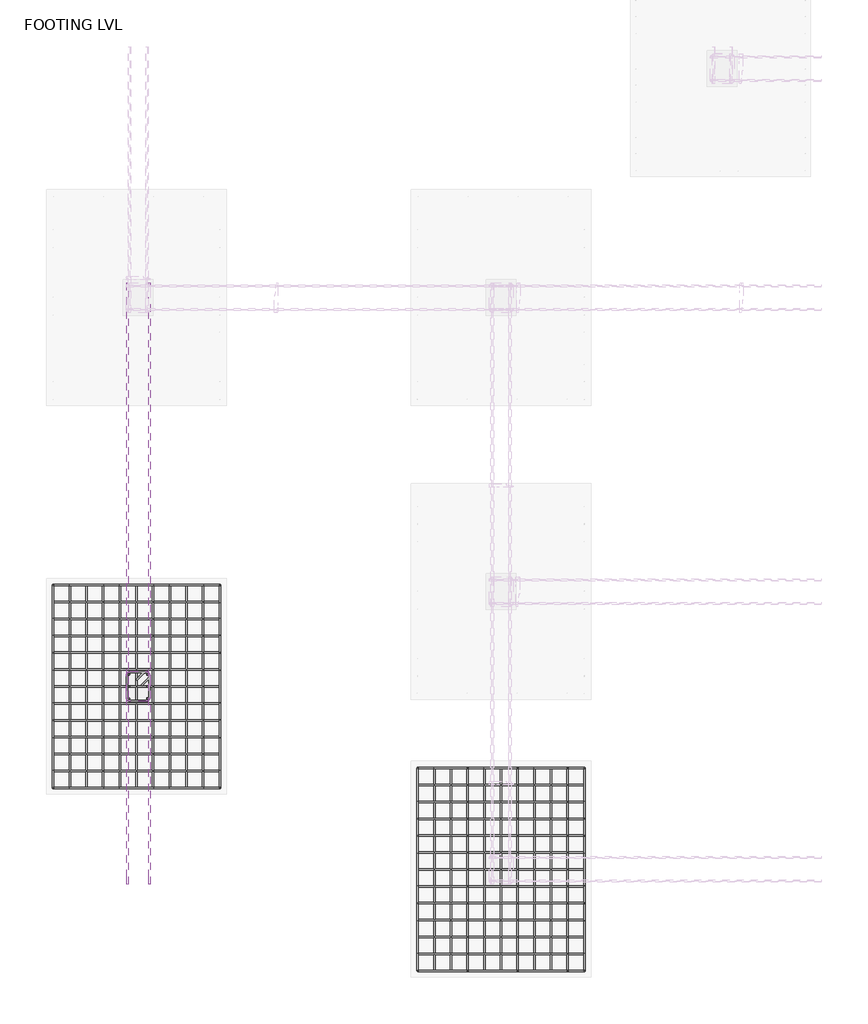
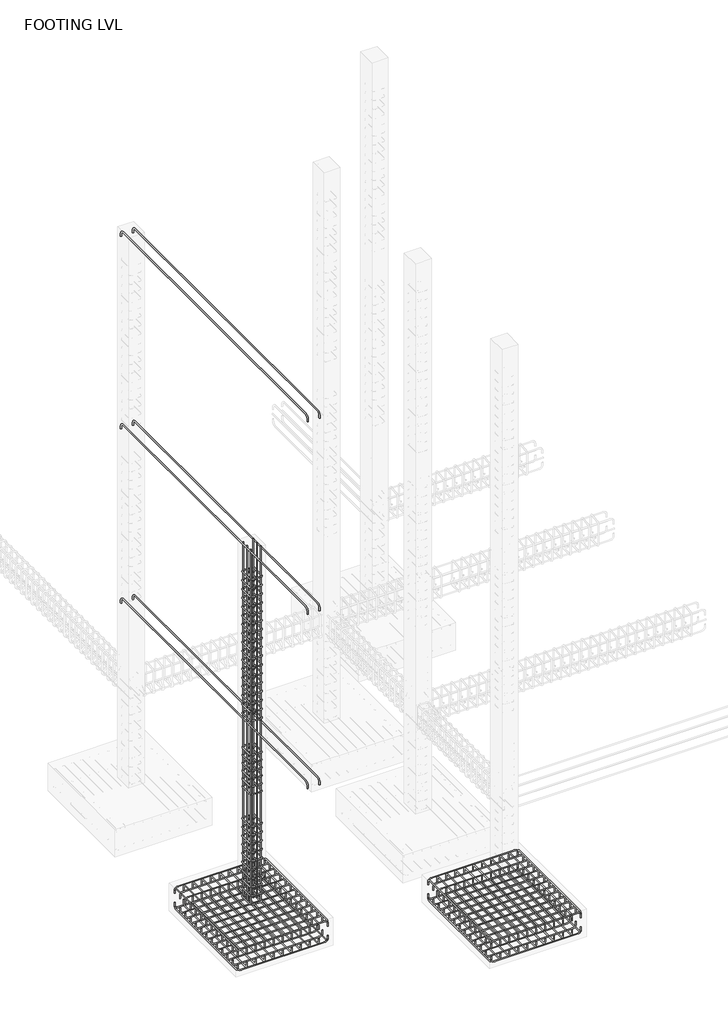
# One storey, part 2 of 16: 23 reinforcing bars.
"""IFC4 building model written with IfcOpenShell, lengths in millimetres."""

from ifc_helpers import new_model, si_unit, point, frame, origin, place, context, project, spatial, polyline, circle_curve, trimmed, segment, composite_curve, source, transform, mapped, element, save
from ifc_brep_helpers import swept_disk

model = new_model("IFC4")

# Units and contexts
model_context = context("Model", 3, world=origin())
ifc_project = project(units=[si_unit("LENGTHUNIT", "METRE", prefix="MILLI")], contexts=[model_context])

# Site, building, storey
site = spatial("IfcSite", under=ifc_project)
building = spatial("IfcBuilding", under=site)
storey = spatial("IfcBuildingStorey", under=building, Name="FOOTING LVL", Elevation=-1828.8)

# Reinforcing bars
placement = place(None, origin())
reinforcing_bar_shape = source(origin(), model_context, "Body", "SolidModel", [
    swept_disk(composite_curve([segment(polyline([(-13401.9759067, 2067.3376269, -2134.39375), (-13401.9759067, 2067.3376269, -2185.19375)]), True, "CONTINUOUS"), segment(trimmed(circle_curve(frame((-13357.5259067, 2067.3376269, -2185.19375), z_axis=(0.0, -1.0, 0.0), x_axis=(-44.44999999999891, 0.0, 0.0)), 44.45), [point((-13401.9759067, 2067.3376269, -2185.19375))], [point((-13357.5259067, 2067.3376269, -2229.64375))], True, "CARTESIAN"), True, "CONTINUOUS"), segment(polyline([(-13357.5259067, 2067.3376269, -2229.64375), (-12035.1384067, 2067.3376269, -2229.64375)]), True, "CONTINUOUS"), segment(trimmed(circle_curve(frame((-12035.1384067, 2067.3376269, -2185.19375), z_axis=(0.0, -1.0, 0.0), x_axis=(0.0, 0.0, -44.45000000000027)), 44.45), [point((-12035.1384067, 2067.3376269, -2229.64375))], [point((-11990.6884067, 2067.3376269, -2185.19375))], True, "CARTESIAN"), True, "CONTINUOUS"), segment(polyline([(-11990.6884067, 2067.3376269, -2185.19375), (-11990.6884067, 2067.3376269, -2134.39375)]), True, "CONTINUOUS")], self_intersect=False), 6.35),
])
element("IfcReinforcingBar", 1, at=placement, inside=storey, context=model_context, shape_type="MappedRepresentation", body=[
    mapped(reinforcing_bar_shape, transform((0.0, 0.0, 0.0), x_axis=(1.0, 0.0, 0.0), y_axis=(0.0, 1.0, 0.0), z_axis=(0.0, 0.0, 1.0))),
    mapped(reinforcing_bar_shape, transform((0.0, 143.0072917, 0.0), x_axis=(1.0, 0.0, 0.0), y_axis=(0.0, 1.0, 0.0), z_axis=(0.0, 0.0, 1.0))),
    mapped(reinforcing_bar_shape, transform((0.0, 286.0145833, 0.0), x_axis=(1.0, 0.0, 0.0), y_axis=(0.0, 1.0, 0.0), z_axis=(0.0, 0.0, 1.0))),
    mapped(reinforcing_bar_shape, transform((0.0, 429.021875, 0.0), x_axis=(1.0, 0.0, 0.0), y_axis=(0.0, 1.0, 0.0), z_axis=(0.0, 0.0, 1.0))),
    mapped(reinforcing_bar_shape, transform((0.0, 572.0291667, 0.0), x_axis=(1.0, 0.0, 0.0), y_axis=(0.0, 1.0, 0.0), z_axis=(0.0, 0.0, 1.0))),
    mapped(reinforcing_bar_shape, transform((0.0, 715.0364583, 0.0), x_axis=(1.0, 0.0, 0.0), y_axis=(0.0, 1.0, 0.0), z_axis=(0.0, 0.0, 1.0))),
    mapped(reinforcing_bar_shape, transform((0.0, 858.04375, 0.0), x_axis=(1.0, 0.0, 0.0), y_axis=(0.0, 1.0, 0.0), z_axis=(0.0, 0.0, 1.0))),
    mapped(reinforcing_bar_shape, transform((0.0, 1001.0510417, 0.0), x_axis=(1.0, 0.0, 0.0), y_axis=(0.0, 1.0, 0.0), z_axis=(0.0, 0.0, 1.0))),
    mapped(reinforcing_bar_shape, transform((0.0, 1144.0583333, 0.0), x_axis=(1.0, 0.0, 0.0), y_axis=(0.0, 1.0, 0.0), z_axis=(0.0, 0.0, 1.0))),
    mapped(reinforcing_bar_shape, transform((0.0, 1287.065625, 0.0), x_axis=(1.0, 0.0, 0.0), y_axis=(0.0, 1.0, 0.0), z_axis=(0.0, 0.0, 1.0))),
    mapped(reinforcing_bar_shape, transform((0.0, 1430.0729167, 0.0), x_axis=(1.0, 0.0, 0.0), y_axis=(0.0, 1.0, 0.0), z_axis=(0.0, 0.0, 1.0))),
    mapped(reinforcing_bar_shape, transform((0.0, 1573.0802083, 0.0), x_axis=(1.0, 0.0, 0.0), y_axis=(0.0, 1.0, 0.0), z_axis=(0.0, 0.0, 1.0))),
    mapped(reinforcing_bar_shape, transform((0.0, 1716.0875, 0.0), x_axis=(1.0, 0.0, 0.0), y_axis=(0.0, 1.0, 0.0), z_axis=(0.0, 0.0, 1.0))),
])
reinforcing_bar_2_shape = source(origin(), model_context, "Body", "SolidModel", [
    swept_disk(composite_curve([segment(polyline([(-11990.6884067, 2067.3376269, -1980.40625), (-11990.6884067, 2067.3376269, -1929.60625)]), True, "CONTINUOUS"), segment(trimmed(circle_curve(frame((-12035.1384067, 2067.3376269, -1929.60625), z_axis=(0.0, -1.0, 0.0), x_axis=(44.45000000000073, 0.0, 0.0)), 44.45), [point((-11990.6884067, 2067.3376269, -1929.60625))], [point((-12035.1384067, 2067.3376269, -1885.15625))], True, "CARTESIAN"), True, "CONTINUOUS"), segment(polyline([(-12035.1384067, 2067.3376269, -1885.15625), (-13357.5259067, 2067.3376269, -1885.15625)]), True, "CONTINUOUS"), segment(trimmed(circle_curve(frame((-13357.5259067, 2067.3376269, -1929.60625), z_axis=(0.0, -1.0, 0.0), x_axis=(0.0, 0.0, 44.450000000000045)), 44.45), [point((-13357.5259067, 2067.3376269, -1885.15625))], [point((-13401.9759067, 2067.3376269, -1929.60625))], True, "CARTESIAN"), True, "CONTINUOUS"), segment(polyline([(-13401.9759067, 2067.3376269, -1929.60625), (-13401.9759067, 2067.3376269, -1980.40625)]), True, "CONTINUOUS")], self_intersect=False), 6.35),
])
element("IfcReinforcingBar", 2, at=placement, inside=storey, context=model_context, shape_type="MappedRepresentation", body=[
    mapped(reinforcing_bar_2_shape, transform((0.0, 0.0, 0.0), x_axis=(1.0, 0.0, 0.0), y_axis=(0.0, 1.0, 0.0), z_axis=(0.0, 0.0, 1.0))),
    mapped(reinforcing_bar_2_shape, transform((0.0, 143.0072917, 0.0), x_axis=(1.0, 0.0, 0.0), y_axis=(0.0, 1.0, 0.0), z_axis=(0.0, 0.0, 1.0))),
    mapped(reinforcing_bar_2_shape, transform((0.0, 286.0145833, 0.0), x_axis=(1.0, 0.0, 0.0), y_axis=(0.0, 1.0, 0.0), z_axis=(0.0, 0.0, 1.0))),
    mapped(reinforcing_bar_2_shape, transform((0.0, 429.021875, 0.0), x_axis=(1.0, 0.0, 0.0), y_axis=(0.0, 1.0, 0.0), z_axis=(0.0, 0.0, 1.0))),
    mapped(reinforcing_bar_2_shape, transform((0.0, 572.0291667, 0.0), x_axis=(1.0, 0.0, 0.0), y_axis=(0.0, 1.0, 0.0), z_axis=(0.0, 0.0, 1.0))),
    mapped(reinforcing_bar_2_shape, transform((0.0, 715.0364583, 0.0), x_axis=(1.0, 0.0, 0.0), y_axis=(0.0, 1.0, 0.0), z_axis=(0.0, 0.0, 1.0))),
    mapped(reinforcing_bar_2_shape, transform((0.0, 858.04375, 0.0), x_axis=(1.0, 0.0, 0.0), y_axis=(0.0, 1.0, 0.0), z_axis=(0.0, 0.0, 1.0))),
    mapped(reinforcing_bar_2_shape, transform((0.0, 1001.0510417, 0.0), x_axis=(1.0, 0.0, 0.0), y_axis=(0.0, 1.0, 0.0), z_axis=(0.0, 0.0, 1.0))),
    mapped(reinforcing_bar_2_shape, transform((0.0, 1144.0583333, 0.0), x_axis=(1.0, 0.0, 0.0), y_axis=(0.0, 1.0, 0.0), z_axis=(0.0, 0.0, 1.0))),
    mapped(reinforcing_bar_2_shape, transform((0.0, 1287.065625, 0.0), x_axis=(1.0, 0.0, 0.0), y_axis=(0.0, 1.0, 0.0), z_axis=(0.0, 0.0, 1.0))),
    mapped(reinforcing_bar_2_shape, transform((0.0, 1430.0729167, 0.0), x_axis=(1.0, 0.0, 0.0), y_axis=(0.0, 1.0, 0.0), z_axis=(0.0, 0.0, 1.0))),
    mapped(reinforcing_bar_2_shape, transform((0.0, 1573.0802083, 0.0), x_axis=(1.0, 0.0, 0.0), y_axis=(0.0, 1.0, 0.0), z_axis=(0.0, 0.0, 1.0))),
    mapped(reinforcing_bar_2_shape, transform((0.0, 1716.0875, 0.0), x_axis=(1.0, 0.0, 0.0), y_axis=(0.0, 1.0, 0.0), z_axis=(0.0, 0.0, 1.0))),
])
reinforcing_bar_3_shape = source(origin(), model_context, "Body", "SolidModel", [
    swept_disk(composite_curve([segment(polyline([(-11990.6884067, 3783.4251269, -1980.40625), (-11990.6884067, 3783.4251269, -1929.60625)]), True, "CONTINUOUS"), segment(trimmed(circle_curve(frame((-11990.6884067, 3738.9751269, -1929.60625), z_axis=(1.0, 0.0, 0.0), x_axis=(0.0, 44.45000000000027, 0.0)), 44.45), [point((-11990.6884067, 3783.4251269, -1929.60625))], [point((-11990.6884067, 3738.9751269, -1885.15625))], True, "CARTESIAN"), True, "CONTINUOUS"), segment(polyline([(-11990.6884067, 3738.9751269, -1885.15625), (-11990.6884067, 2111.7876269, -1885.15625)]), True, "CONTINUOUS"), segment(trimmed(circle_curve(frame((-11990.6884067, 2111.7876269, -1929.60625), z_axis=(1.0, 0.0, 0.0), x_axis=(0.0, 0.0, 44.450000000000045)), 44.45), [point((-11990.6884067, 2111.7876269, -1885.15625))], [point((-11990.6884067, 2067.3376269, -1929.60625))], True, "CARTESIAN"), True, "CONTINUOUS"), segment(polyline([(-11990.6884067, 2067.3376269, -1929.60625), (-11990.6884067, 2067.3376269, -1980.40625)]), True, "CONTINUOUS")], self_intersect=False), 6.35),
])
element("IfcReinforcingBar", 3, at=placement, inside=storey, context=model_context, shape_type="MappedRepresentation", body=[
    mapped(reinforcing_bar_3_shape, transform((0.0, 0.0, 0.0), x_axis=(1.0, 0.0, 0.0), y_axis=(0.0, 1.0, 0.0), z_axis=(0.0, 0.0, 1.0))),
    mapped(reinforcing_bar_3_shape, transform((-141.12875, 0.0, 0.0), x_axis=(1.0, 0.0, 0.0), y_axis=(0.0, 1.0, 0.0), z_axis=(0.0, 0.0, 1.0))),
    mapped(reinforcing_bar_3_shape, transform((-282.2575, 0.0, 0.0), x_axis=(1.0, 0.0, 0.0), y_axis=(0.0, 1.0, 0.0), z_axis=(0.0, 0.0, 1.0))),
    mapped(reinforcing_bar_3_shape, transform((-423.38625, 0.0, 0.0), x_axis=(1.0, 0.0, 0.0), y_axis=(0.0, 1.0, 0.0), z_axis=(0.0, 0.0, 1.0))),
    mapped(reinforcing_bar_3_shape, transform((-564.515, 0.0, 0.0), x_axis=(1.0, 0.0, 0.0), y_axis=(0.0, 1.0, 0.0), z_axis=(0.0, 0.0, 1.0))),
    mapped(reinforcing_bar_3_shape, transform((-705.64375, 0.0, 0.0), x_axis=(1.0, 0.0, 0.0), y_axis=(0.0, 1.0, 0.0), z_axis=(0.0, 0.0, 1.0))),
    mapped(reinforcing_bar_3_shape, transform((-846.7725, 0.0, 0.0), x_axis=(1.0, 0.0, 0.0), y_axis=(0.0, 1.0, 0.0), z_axis=(0.0, 0.0, 1.0))),
    mapped(reinforcing_bar_3_shape, transform((-987.90125, 0.0, 0.0), x_axis=(1.0, 0.0, 0.0), y_axis=(0.0, 1.0, 0.0), z_axis=(0.0, 0.0, 1.0))),
    mapped(reinforcing_bar_3_shape, transform((-1129.03, 0.0, 0.0), x_axis=(1.0, 0.0, 0.0), y_axis=(0.0, 1.0, 0.0), z_axis=(0.0, 0.0, 1.0))),
    mapped(reinforcing_bar_3_shape, transform((-1270.15875, 0.0, 0.0), x_axis=(1.0, 0.0, 0.0), y_axis=(0.0, 1.0, 0.0), z_axis=(0.0, 0.0, 1.0))),
    mapped(reinforcing_bar_3_shape, transform((-1411.2875, 0.0, 0.0), x_axis=(1.0, 0.0, 0.0), y_axis=(0.0, 1.0, 0.0), z_axis=(0.0, 0.0, 1.0))),
])
reinforcing_bar_4_shape = source(origin(), model_context, "Body", "SolidModel", [
    swept_disk(composite_curve([segment(polyline([(-13401.9759067, 3783.4251269, -2134.39375), (-13401.9759067, 3783.4251269, -2185.19375)]), True, "CONTINUOUS"), segment(trimmed(circle_curve(frame((-13401.9759067, 3738.9751269, -2185.19375), z_axis=(-1.0, 0.0, 0.0), x_axis=(0.0, 44.45000000000027, 0.0)), 44.45), [point((-13401.9759067, 3783.4251269, -2185.19375))], [point((-13401.9759067, 3738.9751269, -2229.64375))], True, "CARTESIAN"), True, "CONTINUOUS"), segment(polyline([(-13401.9759067, 3738.9751269, -2229.64375), (-13401.9759067, 2111.7876269, -2229.64375)]), True, "CONTINUOUS"), segment(trimmed(circle_curve(frame((-13401.9759067, 2111.7876269, -2185.19375), z_axis=(-1.0, 0.0, 0.0), x_axis=(0.0, 0.0, -44.45000000000027)), 44.45), [point((-13401.9759067, 2111.7876269, -2229.64375))], [point((-13401.9759067, 2067.3376269, -2185.19375))], True, "CARTESIAN"), True, "CONTINUOUS"), segment(polyline([(-13401.9759067, 2067.3376269, -2185.19375), (-13401.9759067, 2067.3376269, -2134.39375)]), True, "CONTINUOUS")], self_intersect=False), 6.35),
])
element("IfcReinforcingBar", 4, at=placement, inside=storey, context=model_context, shape_type="MappedRepresentation", body=[
    mapped(reinforcing_bar_4_shape, transform((0.0, 0.0, 0.0), x_axis=(1.0, 0.0, 0.0), y_axis=(0.0, 1.0, 0.0), z_axis=(0.0, 0.0, 1.0))),
    mapped(reinforcing_bar_4_shape, transform((141.12875, 0.0, 0.0), x_axis=(1.0, 0.0, 0.0), y_axis=(0.0, 1.0, 0.0), z_axis=(0.0, 0.0, 1.0))),
    mapped(reinforcing_bar_4_shape, transform((282.2575, 0.0, 0.0), x_axis=(1.0, 0.0, 0.0), y_axis=(0.0, 1.0, 0.0), z_axis=(0.0, 0.0, 1.0))),
    mapped(reinforcing_bar_4_shape, transform((423.38625, 0.0, 0.0), x_axis=(1.0, 0.0, 0.0), y_axis=(0.0, 1.0, 0.0), z_axis=(0.0, 0.0, 1.0))),
    mapped(reinforcing_bar_4_shape, transform((564.515, 0.0, 0.0), x_axis=(1.0, 0.0, 0.0), y_axis=(0.0, 1.0, 0.0), z_axis=(0.0, 0.0, 1.0))),
    mapped(reinforcing_bar_4_shape, transform((705.64375, 0.0, 0.0), x_axis=(1.0, 0.0, 0.0), y_axis=(0.0, 1.0, 0.0), z_axis=(0.0, 0.0, 1.0))),
    mapped(reinforcing_bar_4_shape, transform((846.7725, 0.0, 0.0), x_axis=(1.0, 0.0, 0.0), y_axis=(0.0, 1.0, 0.0), z_axis=(0.0, 0.0, 1.0))),
    mapped(reinforcing_bar_4_shape, transform((987.90125, 0.0, 0.0), x_axis=(1.0, 0.0, 0.0), y_axis=(0.0, 1.0, 0.0), z_axis=(0.0, 0.0, 1.0))),
    mapped(reinforcing_bar_4_shape, transform((1129.03, 0.0, 0.0), x_axis=(1.0, 0.0, 0.0), y_axis=(0.0, 1.0, 0.0), z_axis=(0.0, 0.0, 1.0))),
    mapped(reinforcing_bar_4_shape, transform((1270.15875, 0.0, 0.0), x_axis=(1.0, 0.0, 0.0), y_axis=(0.0, 1.0, 0.0), z_axis=(0.0, 0.0, 1.0))),
    mapped(reinforcing_bar_4_shape, transform((1411.2875, 0.0, 0.0), x_axis=(1.0, 0.0, 0.0), y_axis=(0.0, 1.0, 0.0), z_axis=(0.0, 0.0, 1.0))),
])
reinforcing_bar_5_shape = source(origin(), model_context, "Body", "SolidModel", [
    swept_disk(composite_curve([segment(polyline([(-10315.1165072, 517.9376269, -2134.39375), (-10315.1165072, 517.9376269, -2185.19375)]), True, "CONTINUOUS"), segment(trimmed(circle_curve(frame((-10270.6665072, 517.9376269, -2185.19375), z_axis=(0.0, -1.0, 0.0), x_axis=(-44.45000000000073, 0.0, 0.0)), 44.45), [point((-10315.1165072, 517.9376269, -2185.19375))], [point((-10270.6665072, 517.9376269, -2229.64375))], True, "CARTESIAN"), True, "CONTINUOUS"), segment(polyline([(-10270.6665072, 517.9376269, -2229.64375), (-8948.2790072, 517.9376269, -2229.64375)]), True, "CONTINUOUS"), segment(trimmed(circle_curve(frame((-8948.2790072, 517.9376269, -2185.19375), z_axis=(0.0, -1.0, 0.0), x_axis=(0.0, 0.0, -44.45000000000027)), 44.45), [point((-8948.2790072, 517.9376269, -2229.64375))], [point((-8903.8290072, 517.9376269, -2185.19375))], True, "CARTESIAN"), True, "CONTINUOUS"), segment(polyline([(-8903.8290072, 517.9376269, -2185.19375), (-8903.8290072, 517.9376269, -2134.39375)]), True, "CONTINUOUS")], self_intersect=False), 6.35),
])
element("IfcReinforcingBar", 5, at=placement, inside=storey, context=model_context, shape_type="MappedRepresentation", body=[
    mapped(reinforcing_bar_5_shape, transform((0.0, 0.0, 0.0), x_axis=(1.0, 0.0, 0.0), y_axis=(0.0, 1.0, 0.0), z_axis=(0.0, 0.0, 1.0))),
    mapped(reinforcing_bar_5_shape, transform((0.0, 143.0072917, 0.0), x_axis=(1.0, 0.0, 0.0), y_axis=(0.0, 1.0, 0.0), z_axis=(0.0, 0.0, 1.0))),
    mapped(reinforcing_bar_5_shape, transform((0.0, 286.0145833, 0.0), x_axis=(1.0, 0.0, 0.0), y_axis=(0.0, 1.0, 0.0), z_axis=(0.0, 0.0, 1.0))),
    mapped(reinforcing_bar_5_shape, transform((0.0, 429.021875, 0.0), x_axis=(1.0, 0.0, 0.0), y_axis=(0.0, 1.0, 0.0), z_axis=(0.0, 0.0, 1.0))),
    mapped(reinforcing_bar_5_shape, transform((0.0, 572.0291667, 0.0), x_axis=(1.0, 0.0, 0.0), y_axis=(0.0, 1.0, 0.0), z_axis=(0.0, 0.0, 1.0))),
    mapped(reinforcing_bar_5_shape, transform((0.0, 715.0364583, 0.0), x_axis=(1.0, 0.0, 0.0), y_axis=(0.0, 1.0, 0.0), z_axis=(0.0, 0.0, 1.0))),
    mapped(reinforcing_bar_5_shape, transform((0.0, 858.04375, 0.0), x_axis=(1.0, 0.0, 0.0), y_axis=(0.0, 1.0, 0.0), z_axis=(0.0, 0.0, 1.0))),
    mapped(reinforcing_bar_5_shape, transform((0.0, 1001.0510417, 0.0), x_axis=(1.0, 0.0, 0.0), y_axis=(0.0, 1.0, 0.0), z_axis=(0.0, 0.0, 1.0))),
    mapped(reinforcing_bar_5_shape, transform((0.0, 1144.0583333, 0.0), x_axis=(1.0, 0.0, 0.0), y_axis=(0.0, 1.0, 0.0), z_axis=(0.0, 0.0, 1.0))),
    mapped(reinforcing_bar_5_shape, transform((0.0, 1287.065625, 0.0), x_axis=(1.0, 0.0, 0.0), y_axis=(0.0, 1.0, 0.0), z_axis=(0.0, 0.0, 1.0))),
    mapped(reinforcing_bar_5_shape, transform((0.0, 1430.0729167, 0.0), x_axis=(1.0, 0.0, 0.0), y_axis=(0.0, 1.0, 0.0), z_axis=(0.0, 0.0, 1.0))),
    mapped(reinforcing_bar_5_shape, transform((0.0, 1573.0802083, 0.0), x_axis=(1.0, 0.0, 0.0), y_axis=(0.0, 1.0, 0.0), z_axis=(0.0, 0.0, 1.0))),
    mapped(reinforcing_bar_5_shape, transform((0.0, 1716.0875, 0.0), x_axis=(1.0, 0.0, 0.0), y_axis=(0.0, 1.0, 0.0), z_axis=(0.0, 0.0, 1.0))),
])
reinforcing_bar_6_shape = source(origin(), model_context, "Body", "SolidModel", [
    swept_disk(composite_curve([segment(polyline([(-8903.8290072, 517.9376269, -1980.40625), (-8903.8290072, 517.9376269, -1929.60625)]), True, "CONTINUOUS"), segment(trimmed(circle_curve(frame((-8948.2790072, 517.9376269, -1929.60625), z_axis=(0.0, -1.0, 0.0), x_axis=(44.45000000000073, 0.0, 0.0)), 44.45), [point((-8903.8290072, 517.9376269, -1929.60625))], [point((-8948.2790072, 517.9376269, -1885.15625))], True, "CARTESIAN"), True, "CONTINUOUS"), segment(polyline([(-8948.2790072, 517.9376269, -1885.15625), (-10270.6665072, 517.9376269, -1885.15625)]), True, "CONTINUOUS"), segment(trimmed(circle_curve(frame((-10270.6665072, 517.9376269, -1929.60625), z_axis=(0.0, -1.0, 0.0), x_axis=(0.0, 0.0, 44.450000000000045)), 44.45), [point((-10270.6665072, 517.9376269, -1885.15625))], [point((-10315.1165072, 517.9376269, -1929.60625))], True, "CARTESIAN"), True, "CONTINUOUS"), segment(polyline([(-10315.1165072, 517.9376269, -1929.60625), (-10315.1165072, 517.9376269, -1980.40625)]), True, "CONTINUOUS")], self_intersect=False), 6.35),
])
element("IfcReinforcingBar", 6, at=placement, inside=storey, context=model_context, shape_type="MappedRepresentation", body=[
    mapped(reinforcing_bar_6_shape, transform((0.0, 0.0, 0.0), x_axis=(1.0, 0.0, 0.0), y_axis=(0.0, 1.0, 0.0), z_axis=(0.0, 0.0, 1.0))),
    mapped(reinforcing_bar_6_shape, transform((0.0, 143.0072917, 0.0), x_axis=(1.0, 0.0, 0.0), y_axis=(0.0, 1.0, 0.0), z_axis=(0.0, 0.0, 1.0))),
    mapped(reinforcing_bar_6_shape, transform((0.0, 286.0145833, 0.0), x_axis=(1.0, 0.0, 0.0), y_axis=(0.0, 1.0, 0.0), z_axis=(0.0, 0.0, 1.0))),
    mapped(reinforcing_bar_6_shape, transform((0.0, 429.021875, 0.0), x_axis=(1.0, 0.0, 0.0), y_axis=(0.0, 1.0, 0.0), z_axis=(0.0, 0.0, 1.0))),
    mapped(reinforcing_bar_6_shape, transform((0.0, 572.0291667, 0.0), x_axis=(1.0, 0.0, 0.0), y_axis=(0.0, 1.0, 0.0), z_axis=(0.0, 0.0, 1.0))),
    mapped(reinforcing_bar_6_shape, transform((0.0, 715.0364583, 0.0), x_axis=(1.0, 0.0, 0.0), y_axis=(0.0, 1.0, 0.0), z_axis=(0.0, 0.0, 1.0))),
    mapped(reinforcing_bar_6_shape, transform((0.0, 858.04375, 0.0), x_axis=(1.0, 0.0, 0.0), y_axis=(0.0, 1.0, 0.0), z_axis=(0.0, 0.0, 1.0))),
    mapped(reinforcing_bar_6_shape, transform((0.0, 1001.0510417, 0.0), x_axis=(1.0, 0.0, 0.0), y_axis=(0.0, 1.0, 0.0), z_axis=(0.0, 0.0, 1.0))),
    mapped(reinforcing_bar_6_shape, transform((0.0, 1144.0583333, 0.0), x_axis=(1.0, 0.0, 0.0), y_axis=(0.0, 1.0, 0.0), z_axis=(0.0, 0.0, 1.0))),
    mapped(reinforcing_bar_6_shape, transform((0.0, 1287.065625, 0.0), x_axis=(1.0, 0.0, 0.0), y_axis=(0.0, 1.0, 0.0), z_axis=(0.0, 0.0, 1.0))),
    mapped(reinforcing_bar_6_shape, transform((0.0, 1430.0729167, 0.0), x_axis=(1.0, 0.0, 0.0), y_axis=(0.0, 1.0, 0.0), z_axis=(0.0, 0.0, 1.0))),
    mapped(reinforcing_bar_6_shape, transform((0.0, 1573.0802083, 0.0), x_axis=(1.0, 0.0, 0.0), y_axis=(0.0, 1.0, 0.0), z_axis=(0.0, 0.0, 1.0))),
    mapped(reinforcing_bar_6_shape, transform((0.0, 1716.0875, 0.0), x_axis=(1.0, 0.0, 0.0), y_axis=(0.0, 1.0, 0.0), z_axis=(0.0, 0.0, 1.0))),
])
reinforcing_bar_7_shape = source(origin(), model_context, "Body", "SolidModel", [
    swept_disk(composite_curve([segment(polyline([(-8903.8290072, 2234.0251269, -1980.40625), (-8903.8290072, 2234.0251269, -1929.60625)]), True, "CONTINUOUS"), segment(trimmed(circle_curve(frame((-8903.8290072, 2189.5751269, -1929.60625), z_axis=(1.0, 0.0, 0.0), x_axis=(0.0, 44.44999999999982, 0.0)), 44.45), [point((-8903.8290072, 2234.0251269, -1929.60625))], [point((-8903.8290072, 2189.5751269, -1885.15625))], True, "CARTESIAN"), True, "CONTINUOUS"), segment(polyline([(-8903.8290072, 2189.5751269, -1885.15625), (-8903.8290072, 562.3876269, -1885.15625)]), True, "CONTINUOUS"), segment(trimmed(circle_curve(frame((-8903.8290072, 562.3876269, -1929.60625), z_axis=(1.0, 0.0, 0.0), x_axis=(0.0, 0.0, 44.450000000000045)), 44.45), [point((-8903.8290072, 562.3876269, -1885.15625))], [point((-8903.8290072, 517.9376269, -1929.60625))], True, "CARTESIAN"), True, "CONTINUOUS"), segment(polyline([(-8903.8290072, 517.9376269, -1929.60625), (-8903.8290072, 517.9376269, -1980.40625)]), True, "CONTINUOUS")], self_intersect=False), 6.35),
])
element("IfcReinforcingBar", 7, at=placement, inside=storey, context=model_context, shape_type="MappedRepresentation", body=[
    mapped(reinforcing_bar_7_shape, transform((0.0, 0.0, 0.0), x_axis=(1.0, 0.0, 0.0), y_axis=(0.0, 1.0, 0.0), z_axis=(0.0, 0.0, 1.0))),
    mapped(reinforcing_bar_7_shape, transform((-141.12875, 0.0, 0.0), x_axis=(1.0, 0.0, 0.0), y_axis=(0.0, 1.0, 0.0), z_axis=(0.0, 0.0, 1.0))),
    mapped(reinforcing_bar_7_shape, transform((-282.2575, 0.0, 0.0), x_axis=(1.0, 0.0, 0.0), y_axis=(0.0, 1.0, 0.0), z_axis=(0.0, 0.0, 1.0))),
    mapped(reinforcing_bar_7_shape, transform((-423.38625, 0.0, 0.0), x_axis=(1.0, 0.0, 0.0), y_axis=(0.0, 1.0, 0.0), z_axis=(0.0, 0.0, 1.0))),
    mapped(reinforcing_bar_7_shape, transform((-564.515, 0.0, 0.0), x_axis=(1.0, 0.0, 0.0), y_axis=(0.0, 1.0, 0.0), z_axis=(0.0, 0.0, 1.0))),
    mapped(reinforcing_bar_7_shape, transform((-705.64375, 0.0, 0.0), x_axis=(1.0, 0.0, 0.0), y_axis=(0.0, 1.0, 0.0), z_axis=(0.0, 0.0, 1.0))),
    mapped(reinforcing_bar_7_shape, transform((-846.7725, 0.0, 0.0), x_axis=(1.0, 0.0, 0.0), y_axis=(0.0, 1.0, 0.0), z_axis=(0.0, 0.0, 1.0))),
    mapped(reinforcing_bar_7_shape, transform((-987.90125, 0.0, 0.0), x_axis=(1.0, 0.0, 0.0), y_axis=(0.0, 1.0, 0.0), z_axis=(0.0, 0.0, 1.0))),
    mapped(reinforcing_bar_7_shape, transform((-1129.03, 0.0, 0.0), x_axis=(1.0, 0.0, 0.0), y_axis=(0.0, 1.0, 0.0), z_axis=(0.0, 0.0, 1.0))),
    mapped(reinforcing_bar_7_shape, transform((-1270.15875, 0.0, 0.0), x_axis=(1.0, 0.0, 0.0), y_axis=(0.0, 1.0, 0.0), z_axis=(0.0, 0.0, 1.0))),
    mapped(reinforcing_bar_7_shape, transform((-1411.2875, 0.0, 0.0), x_axis=(1.0, 0.0, 0.0), y_axis=(0.0, 1.0, 0.0), z_axis=(0.0, 0.0, 1.0))),
])
reinforcing_bar_8_shape = source(origin(), model_context, "Body", "SolidModel", [
    swept_disk(composite_curve([segment(polyline([(-10315.1165072, 2234.0251269, -2134.39375), (-10315.1165072, 2234.0251269, -2185.19375)]), True, "CONTINUOUS"), segment(trimmed(circle_curve(frame((-10315.1165072, 2189.5751269, -2185.19375), z_axis=(-1.0, 0.0, 0.0), x_axis=(0.0, 44.44999999999982, 0.0)), 44.45), [point((-10315.1165072, 2234.0251269, -2185.19375))], [point((-10315.1165072, 2189.5751269, -2229.64375))], True, "CARTESIAN"), True, "CONTINUOUS"), segment(polyline([(-10315.1165072, 2189.5751269, -2229.64375), (-10315.1165072, 562.3876269, -2229.64375)]), True, "CONTINUOUS"), segment(trimmed(circle_curve(frame((-10315.1165072, 562.3876269, -2185.19375), z_axis=(-1.0, 0.0, 0.0), x_axis=(0.0, 0.0, -44.45000000000027)), 44.45), [point((-10315.1165072, 562.3876269, -2229.64375))], [point((-10315.1165072, 517.9376269, -2185.19375))], True, "CARTESIAN"), True, "CONTINUOUS"), segment(polyline([(-10315.1165072, 517.9376269, -2185.19375), (-10315.1165072, 517.9376269, -2134.39375)]), True, "CONTINUOUS")], self_intersect=False), 6.35),
])
element("IfcReinforcingBar", 8, at=placement, inside=storey, context=model_context, shape_type="MappedRepresentation", body=[
    mapped(reinforcing_bar_8_shape, transform((0.0, 0.0, 0.0), x_axis=(1.0, 0.0, 0.0), y_axis=(0.0, 1.0, 0.0), z_axis=(0.0, 0.0, 1.0))),
    mapped(reinforcing_bar_8_shape, transform((141.12875, 0.0, 0.0), x_axis=(1.0, 0.0, 0.0), y_axis=(0.0, 1.0, 0.0), z_axis=(0.0, 0.0, 1.0))),
    mapped(reinforcing_bar_8_shape, transform((282.2575, 0.0, 0.0), x_axis=(1.0, 0.0, 0.0), y_axis=(0.0, 1.0, 0.0), z_axis=(0.0, 0.0, 1.0))),
    mapped(reinforcing_bar_8_shape, transform((423.38625, 0.0, 0.0), x_axis=(1.0, 0.0, 0.0), y_axis=(0.0, 1.0, 0.0), z_axis=(0.0, 0.0, 1.0))),
    mapped(reinforcing_bar_8_shape, transform((564.515, 0.0, 0.0), x_axis=(1.0, 0.0, 0.0), y_axis=(0.0, 1.0, 0.0), z_axis=(0.0, 0.0, 1.0))),
    mapped(reinforcing_bar_8_shape, transform((705.64375, 0.0, 0.0), x_axis=(1.0, 0.0, 0.0), y_axis=(0.0, 1.0, 0.0), z_axis=(0.0, 0.0, 1.0))),
    mapped(reinforcing_bar_8_shape, transform((846.7725, 0.0, 0.0), x_axis=(1.0, 0.0, 0.0), y_axis=(0.0, 1.0, 0.0), z_axis=(0.0, 0.0, 1.0))),
    mapped(reinforcing_bar_8_shape, transform((987.90125, 0.0, 0.0), x_axis=(1.0, 0.0, 0.0), y_axis=(0.0, 1.0, 0.0), z_axis=(0.0, 0.0, 1.0))),
    mapped(reinforcing_bar_8_shape, transform((1129.03, 0.0, 0.0), x_axis=(1.0, 0.0, 0.0), y_axis=(0.0, 1.0, 0.0), z_axis=(0.0, 0.0, 1.0))),
    mapped(reinforcing_bar_8_shape, transform((1270.15875, 0.0, 0.0), x_axis=(1.0, 0.0, 0.0), y_axis=(0.0, 1.0, 0.0), z_axis=(0.0, 0.0, 1.0))),
    mapped(reinforcing_bar_8_shape, transform((1411.2875, 0.0, 0.0), x_axis=(1.0, 0.0, 0.0), y_axis=(0.0, 1.0, 0.0), z_axis=(0.0, 0.0, 1.0))),
])
element("IfcReinforcingBar", 9, at=placement, inside=storey, context=model_context, shape_type="SolidModel", body=[
    swept_disk(composite_curve([segment(polyline([(-12773.3602572, 6336.1637461, 7172.721875), (-12773.3602572, 6336.1637461, 7210.821875)]), True, "CONTINUOUS"), segment(trimmed(circle_curve(frame((-12773.3602572, 6280.6012461, 7210.821875), z_axis=(1.0, 0.0, 0.0), x_axis=(0.0, 55.5625, 0.0)), 55.5625), [point((-12773.3602572, 6336.1637461, 7210.821875))], [point((-12773.3602572, 6280.6012461, 7266.384375))], True, "CARTESIAN"), True, "CONTINUOUS"), segment(polyline([(-12773.3602572, 6280.6012461, 7266.384375), (-12773.3602572, 1312.0845019, 7266.384375)]), True, "CONTINUOUS"), segment(trimmed(circle_curve(frame((-12773.3602572, 1312.0845019, 7210.821875), z_axis=(1.0, 0.0, 0.0), x_axis=(0.0, 0.0, 55.5625)), 55.5625), [point((-12773.3602572, 1312.0845019, 7266.384375))], [point((-12773.3602572, 1256.5220019, 7210.821875))], True, "CARTESIAN"), True, "CONTINUOUS"), segment(polyline([(-12773.3602572, 1256.5220019, 7210.821875), (-12773.3602572, 1256.5220019, 7172.721875)]), True, "CONTINUOUS")], self_intersect=False), 7.9375),
])
element("IfcReinforcingBar", 10, at=placement, inside=storey, context=model_context, shape_type="SolidModel", body=[
    swept_disk(composite_curve([segment(polyline([(-12586.262902, 6336.1637461, 7165.7473552), (-12586.262902, 6336.1637461, 7203.8473552)]), True, "CONTINUOUS"), segment(trimmed(circle_curve(frame((-12586.262902, 6280.6012461, 7203.8473552), z_axis=(1.0, 0.0, 0.0), x_axis=(0.0, 55.5625, 0.0)), 55.5625), [point((-12586.262902, 6336.1637461, 7203.8473552))], [point((-12586.262902, 6280.6012461, 7259.4098552))], True, "CARTESIAN"), True, "CONTINUOUS"), segment(polyline([(-12586.262902, 6280.6012461, 7259.4098552), (-12586.262902, 1312.0845019, 7259.4098552)]), True, "CONTINUOUS"), segment(trimmed(circle_curve(frame((-12586.262902, 1312.0845019, 7203.8473552), z_axis=(1.0, 0.0, 0.0), x_axis=(0.0, 0.0, 55.5625)), 55.5625), [point((-12586.262902, 1312.0845019, 7259.4098552))], [point((-12586.262902, 1256.5220019, 7203.8473552))], True, "CARTESIAN"), True, "CONTINUOUS"), segment(polyline([(-12586.262902, 1256.5220019, 7203.8473552), (-12586.262902, 1256.5220019, 7165.7473552)]), True, "CONTINUOUS")], self_intersect=False), 7.9375),
])
reinforcing_bar_9_shape = source(origin(), model_context, "Body", "SolidModel", [
    swept_disk(composite_curve([segment(polyline([(-12651.3902404, 2937.3626131, -1797.446875), (-12596.5252419, 2992.2276116, -1797.446875)]), True, "CONTINUOUS"), segment(trimmed(circle_curve(frame((-12618.9758822, 3014.6782519, -1797.446875), z_axis=(0.0, 0.0, 1.0), x_axis=(22.450640299999577, -22.450640300000032, 0.0)), 31.75), [point((-12596.5252419, 2992.2276116, -1797.446875))], [point((-12618.9758822, 3046.4282519, -1797.446875))], True, "CARTESIAN"), True, "CONTINUOUS"), segment(polyline([(-12618.9758822, 3046.4282519, -1797.446875), (-12746.7696322, 3046.4282519, -1797.446875)]), True, "CONTINUOUS"), segment(trimmed(circle_curve(frame((-12746.7696322, 3014.6782519, -1797.446875), z_axis=(0.0, 0.0, 1.0), x_axis=(0.0, 31.75, 0.0)), 31.75), [point((-12746.7696322, 3046.4282519, -1797.446875))], [point((-12778.5196322, 3014.6782519, -1797.446875))], True, "CARTESIAN"), True, "CONTINUOUS"), segment(polyline([(-12778.5196322, 3014.6782519, -1797.446875), (-12778.5196322, 2836.0845019, -1797.446875)]), True, "CONTINUOUS"), segment(trimmed(circle_curve(frame((-12746.839373, 2836.0845019, -1799.5501287), z_axis=(0.06624421176864072, 0.0, 0.9978034397651431), x_axis=(-31.680259199998545, 0.0, 2.1032536999998683)), 31.75), [point((-12778.5196322, 2836.0845019, -1797.446875))], [point((-12746.839373, 2804.3345019, -1799.5501287))], True, "CARTESIAN"), True, "CONTINUOUS"), segment(polyline([(-12746.839373, 2804.3345019, -1799.5501287), (-12618.9061414, 2804.3345019, -1808.0436213)]), True, "CONTINUOUS"), segment(trimmed(circle_curve(frame((-12618.9061414, 2836.0845019, -1808.0436213), z_axis=(0.06624421176864072, 0.0, 0.9978034397651431), x_axis=(0.0, -31.75, 0.0)), 31.75), [point((-12618.9061414, 2804.3345019, -1808.0436213))], [point((-12587.2258822, 2836.0845019, -1810.146875))], True, "CARTESIAN"), True, "CONTINUOUS"), segment(polyline([(-12587.2258822, 2836.0845019, -1810.146875), (-12587.2258822, 3014.6782519, -1810.146875)]), True, "CONTINUOUS"), segment(trimmed(circle_curve(frame((-12618.9758822, 3014.6782519, -1810.146875), z_axis=(0.0, 0.0, 1.0), x_axis=(31.75, 0.0, 0.0)), 31.75), [point((-12587.2258822, 3014.6782519, -1810.146875))], [point((-12641.4265225, 3037.1288922, -1810.146875))], True, "CARTESIAN"), True, "CONTINUOUS"), segment(polyline([(-12641.4265225, 3037.1288922, -1810.146875), (-12696.291521, 2982.2638937, -1810.146875)]), True, "CONTINUOUS")], self_intersect=False), 6.35),
])
element("IfcReinforcingBar", 11, at=placement, inside=storey, context=model_context, shape_type="MappedRepresentation", body=[
    mapped(reinforcing_bar_9_shape, transform((0.0, 0.0, 0.0), x_axis=(1.0, 0.0, 0.0), y_axis=(0.0, 1.0, 0.0), z_axis=(0.0, 0.0, 1.0))),
    mapped(reinforcing_bar_9_shape, transform((0.0, 0.0, 144.2276574), x_axis=(1.0, 0.0, 0.0), y_axis=(0.0, 1.0, 0.0), z_axis=(0.0, 0.0, 1.0))),
    mapped(reinforcing_bar_9_shape, transform((0.0, 0.0, 288.4553149), x_axis=(1.0, 0.0, 0.0), y_axis=(0.0, 1.0, 0.0), z_axis=(0.0, 0.0, 1.0))),
    mapped(reinforcing_bar_9_shape, transform((0.0, 0.0, 432.6829723), x_axis=(1.0, 0.0, 0.0), y_axis=(0.0, 1.0, 0.0), z_axis=(0.0, 0.0, 1.0))),
    mapped(reinforcing_bar_9_shape, transform((0.0, 0.0, 576.9106298), x_axis=(1.0, 0.0, 0.0), y_axis=(0.0, 1.0, 0.0), z_axis=(0.0, 0.0, 1.0))),
    mapped(reinforcing_bar_9_shape, transform((0.0, 0.0, 721.1382872), x_axis=(1.0, 0.0, 0.0), y_axis=(0.0, 1.0, 0.0), z_axis=(0.0, 0.0, 1.0))),
    mapped(reinforcing_bar_9_shape, transform((0.0, 0.0, 865.3659446), x_axis=(1.0, 0.0, 0.0), y_axis=(0.0, 1.0, 0.0), z_axis=(0.0, 0.0, 1.0))),
    mapped(reinforcing_bar_9_shape, transform((0.0, 0.0, 1009.5936021), x_axis=(1.0, 0.0, 0.0), y_axis=(0.0, 1.0, 0.0), z_axis=(0.0, 0.0, 1.0))),
    mapped(reinforcing_bar_9_shape, transform((0.0, 0.0, 1153.8212595), x_axis=(1.0, 0.0, 0.0), y_axis=(0.0, 1.0, 0.0), z_axis=(0.0, 0.0, 1.0))),
    mapped(reinforcing_bar_9_shape, transform((0.0, 0.0, 1298.048917), x_axis=(1.0, 0.0, 0.0), y_axis=(0.0, 1.0, 0.0), z_axis=(0.0, 0.0, 1.0))),
])
element("IfcReinforcingBar", 12, at=placement, inside=storey, context=model_context, shape_type="SolidModel", body=[
    swept_disk(composite_curve([segment(polyline([(-12605.505498, 3028.1486361, -1803.796875), (-12605.505498, 3028.1486361, 4089.796875)]), True, "CONTINUOUS")], self_intersect=False), 6.35),
])
element("IfcReinforcingBar", 13, at=placement, inside=storey, context=model_context, shape_type="SolidModel", body=[
    swept_disk(composite_curve([segment(polyline([(-12760.2400164, 3028.1486361, -1803.796875), (-12760.2400164, 3028.1486361, 4089.796875)]), True, "CONTINUOUS")], self_intersect=False), 6.35),
])
element("IfcReinforcingBar", 14, at=placement, inside=storey, context=model_context, shape_type="SolidModel", body=[
    swept_disk(composite_curve([segment(polyline([(-12605.505498, 2822.6141177, -1803.796875), (-12605.505498, 2822.6141177, 4089.796875)]), True, "CONTINUOUS")], self_intersect=False), 6.35),
])
element("IfcReinforcingBar", 15, at=placement, inside=storey, context=model_context, shape_type="SolidModel", body=[
    swept_disk(composite_curve([segment(polyline([(-12760.2400164, 2822.6141177, -1803.796875), (-12760.2400164, 2822.6141177, 4089.796875)]), True, "CONTINUOUS")], self_intersect=False), 6.35),
])
element("IfcReinforcingBar", 16, at=placement, inside=storey, context=model_context, shape_type="SolidModel", body=[
    swept_disk(composite_curve([segment(polyline([(-12605.505498, 2925.3813769, -1803.796875), (-12605.505498, 2925.3813769, 4089.796875)]), True, "CONTINUOUS")], self_intersect=False), 6.35),
])
element("IfcReinforcingBar", 17, at=placement, inside=storey, context=model_context, shape_type="SolidModel", body=[
    swept_disk(composite_curve([segment(polyline([(-12760.2400164, 2925.3813769, -1803.796875), (-12760.2400164, 2925.3813769, 4089.796875)]), True, "CONTINUOUS")], self_intersect=False), 6.35),
])
reinforcing_bar_10_shape = source(origin(), model_context, "Body", "SolidModel", [
    swept_disk(composite_curve([segment(polyline([(-12651.3902404, 2937.3626131, 31.353125), (-12596.5252419, 2992.2276116, 31.353125)]), True, "CONTINUOUS"), segment(trimmed(circle_curve(frame((-12618.9758822, 3014.6782519, 31.353125), z_axis=(0.0, 0.0, 1.0), x_axis=(22.450640299999577, -22.450640300000032, 0.0)), 31.75), [point((-12596.5252419, 2992.2276116, 31.353125))], [point((-12618.9758822, 3046.4282519, 31.353125))], True, "CARTESIAN"), True, "CONTINUOUS"), segment(polyline([(-12618.9758822, 3046.4282519, 31.353125), (-12746.7696322, 3046.4282519, 31.353125)]), True, "CONTINUOUS"), segment(trimmed(circle_curve(frame((-12746.7696322, 3014.6782519, 31.353125), z_axis=(0.0, 0.0, 1.0), x_axis=(0.0, 31.75, 0.0)), 31.75), [point((-12746.7696322, 3046.4282519, 31.353125))], [point((-12778.5196322, 3014.6782519, 31.353125))], True, "CARTESIAN"), True, "CONTINUOUS"), segment(polyline([(-12778.5196322, 3014.6782519, 31.353125), (-12778.5196322, 2836.0845019, 31.353125)]), True, "CONTINUOUS"), segment(trimmed(circle_curve(frame((-12746.839373, 2836.0845019, 29.2498713), z_axis=(0.06624421176864072, 0.0, 0.9978034397651431), x_axis=(-31.680259199998545, 0.0, 2.1032537)), 31.75), [point((-12778.5196322, 2836.0845019, 31.353125))], [point((-12746.839373, 2804.3345019, 29.2498713))], True, "CARTESIAN"), True, "CONTINUOUS"), segment(polyline([(-12746.839373, 2804.3345019, 29.2498713), (-12618.9061414, 2804.3345019, 20.7563787)]), True, "CONTINUOUS"), segment(trimmed(circle_curve(frame((-12618.9061414, 2836.0845019, 20.7563787), z_axis=(0.06624421176864072, 0.0, 0.9978034397651431), x_axis=(0.0, -31.75, 0.0)), 31.75), [point((-12618.9061414, 2804.3345019, 20.7563787))], [point((-12587.2258822, 2836.0845019, 18.653125))], True, "CARTESIAN"), True, "CONTINUOUS"), segment(polyline([(-12587.2258822, 2836.0845019, 18.653125), (-12587.2258822, 3014.6782519, 18.653125)]), True, "CONTINUOUS"), segment(trimmed(circle_curve(frame((-12618.9758822, 3014.6782519, 18.653125), z_axis=(0.0, 0.0, 1.0), x_axis=(31.75, 0.0, 0.0)), 31.75), [point((-12587.2258822, 3014.6782519, 18.653125))], [point((-12641.4265225, 3037.1288922, 18.653125))], True, "CARTESIAN"), True, "CONTINUOUS"), segment(polyline([(-12641.4265225, 3037.1288922, 18.653125), (-12696.291521, 2982.2638937, 18.653125)]), True, "CONTINUOUS")], self_intersect=False), 6.35),
])
element("IfcReinforcingBar", 18, at=placement, inside=storey, context=model_context, shape_type="MappedRepresentation", body=[
    mapped(reinforcing_bar_10_shape, transform((0.0, 0.0, 0.0), x_axis=(1.0, 0.0, 0.0), y_axis=(0.0, 1.0, 0.0), z_axis=(0.0, 0.0, 1.0))),
    mapped(reinforcing_bar_10_shape, transform((0.0, 0.0, 130.6477176), x_axis=(1.0, 0.0, 0.0), y_axis=(0.0, 1.0, 0.0), z_axis=(0.0, 0.0, 1.0))),
    mapped(reinforcing_bar_10_shape, transform((0.0, 0.0, 261.2954352), x_axis=(1.0, 0.0, 0.0), y_axis=(0.0, 1.0, 0.0), z_axis=(0.0, 0.0, 1.0))),
    mapped(reinforcing_bar_10_shape, transform((0.0, 0.0, 391.9431528), x_axis=(1.0, 0.0, 0.0), y_axis=(0.0, 1.0, 0.0), z_axis=(0.0, 0.0, 1.0))),
    mapped(reinforcing_bar_10_shape, transform((0.0, 0.0, 522.5908704), x_axis=(1.0, 0.0, 0.0), y_axis=(0.0, 1.0, 0.0), z_axis=(0.0, 0.0, 1.0))),
    mapped(reinforcing_bar_10_shape, transform((0.0, 0.0, 653.238588), x_axis=(1.0, 0.0, 0.0), y_axis=(0.0, 1.0, 0.0), z_axis=(0.0, 0.0, 1.0))),
])
reinforcing_bar_11_shape = source(origin(), model_context, "Body", "SolidModel", [
    swept_disk(composite_curve([segment(polyline([(-12651.3902404, 2937.3626131, 1250.553125), (-12596.5252419, 2992.2276116, 1250.553125)]), True, "CONTINUOUS"), segment(trimmed(circle_curve(frame((-12618.9758822, 3014.6782519, 1250.553125), z_axis=(0.0, 0.0, 1.0), x_axis=(22.450640299999577, -22.450640300000032, 0.0)), 31.75), [point((-12596.5252419, 2992.2276116, 1250.553125))], [point((-12618.9758822, 3046.4282519, 1250.553125))], True, "CARTESIAN"), True, "CONTINUOUS"), segment(polyline([(-12618.9758822, 3046.4282519, 1250.553125), (-12746.7696322, 3046.4282519, 1250.553125)]), True, "CONTINUOUS"), segment(trimmed(circle_curve(frame((-12746.7696322, 3014.6782519, 1250.553125), z_axis=(0.0, 0.0, 1.0), x_axis=(0.0, 31.75, 0.0)), 31.75), [point((-12746.7696322, 3046.4282519, 1250.553125))], [point((-12778.5196322, 3014.6782519, 1250.553125))], True, "CARTESIAN"), True, "CONTINUOUS"), segment(polyline([(-12778.5196322, 3014.6782519, 1250.553125), (-12778.5196322, 2836.0845019, 1250.553125)]), True, "CONTINUOUS"), segment(trimmed(circle_curve(frame((-12746.839373, 2836.0845019, 1248.4498713), z_axis=(0.06624421176864072, 0.0, 0.9978034397651431), x_axis=(-31.680259199998545, 0.0, 2.1032536999998683)), 31.75), [point((-12778.5196322, 2836.0845019, 1250.553125))], [point((-12746.839373, 2804.3345019, 1248.4498713))], True, "CARTESIAN"), True, "CONTINUOUS"), segment(polyline([(-12746.839373, 2804.3345019, 1248.4498713), (-12618.9061414, 2804.3345019, 1239.9563787)]), True, "CONTINUOUS"), segment(trimmed(circle_curve(frame((-12618.9061414, 2836.0845019, 1239.9563787), z_axis=(0.06624421176864072, 0.0, 0.9978034397651431), x_axis=(0.0, -31.75, 0.0)), 31.75), [point((-12618.9061414, 2804.3345019, 1239.9563787))], [point((-12587.2258822, 2836.0845019, 1237.853125))], True, "CARTESIAN"), True, "CONTINUOUS"), segment(polyline([(-12587.2258822, 2836.0845019, 1237.853125), (-12587.2258822, 3014.6782519, 1237.853125)]), True, "CONTINUOUS"), segment(trimmed(circle_curve(frame((-12618.9758822, 3014.6782519, 1237.853125), z_axis=(0.0, 0.0, 1.0), x_axis=(31.75, 0.0, 0.0)), 31.75), [point((-12587.2258822, 3014.6782519, 1237.853125))], [point((-12641.4265225, 3037.1288922, 1237.853125))], True, "CARTESIAN"), True, "CONTINUOUS"), segment(polyline([(-12641.4265225, 3037.1288922, 1237.853125), (-12696.291521, 2982.2638937, 1237.853125)]), True, "CONTINUOUS")], self_intersect=False), 6.35),
])
element("IfcReinforcingBar", 19, at=placement, inside=storey, context=model_context, shape_type="MappedRepresentation", body=[
    mapped(reinforcing_bar_11_shape, transform((0.0, 0.0, 0.0), x_axis=(1.0, 0.0, 0.0), y_axis=(0.0, 1.0, 0.0), z_axis=(0.0, 0.0, 1.0))),
    mapped(reinforcing_bar_11_shape, transform((0.0, 0.0, 147.1336535), x_axis=(1.0, 0.0, 0.0), y_axis=(0.0, 1.0, 0.0), z_axis=(0.0, 0.0, 1.0))),
    mapped(reinforcing_bar_11_shape, transform((0.0, 0.0, 294.267307), x_axis=(1.0, 0.0, 0.0), y_axis=(0.0, 1.0, 0.0), z_axis=(0.0, 0.0, 1.0))),
    mapped(reinforcing_bar_11_shape, transform((0.0, 0.0, 441.4009605), x_axis=(1.0, 0.0, 0.0), y_axis=(0.0, 1.0, 0.0), z_axis=(0.0, 0.0, 1.0))),
    mapped(reinforcing_bar_11_shape, transform((0.0, 0.0, 588.534614), x_axis=(1.0, 0.0, 0.0), y_axis=(0.0, 1.0, 0.0), z_axis=(0.0, 0.0, 1.0))),
    mapped(reinforcing_bar_11_shape, transform((0.0, 0.0, 735.6682675), x_axis=(1.0, 0.0, 0.0), y_axis=(0.0, 1.0, 0.0), z_axis=(0.0, 0.0, 1.0))),
    mapped(reinforcing_bar_11_shape, transform((0.0, 0.0, 882.801921), x_axis=(1.0, 0.0, 0.0), y_axis=(0.0, 1.0, 0.0), z_axis=(0.0, 0.0, 1.0))),
    mapped(reinforcing_bar_11_shape, transform((0.0, 0.0, 1029.9355745), x_axis=(1.0, 0.0, 0.0), y_axis=(0.0, 1.0, 0.0), z_axis=(0.0, 0.0, 1.0))),
    mapped(reinforcing_bar_11_shape, transform((0.0, 0.0, 1177.069228), x_axis=(1.0, 0.0, 0.0), y_axis=(0.0, 1.0, 0.0), z_axis=(0.0, 0.0, 1.0))),
    mapped(reinforcing_bar_11_shape, transform((0.0, 0.0, 1324.2028815), x_axis=(1.0, 0.0, 0.0), y_axis=(0.0, 1.0, 0.0), z_axis=(0.0, 0.0, 1.0))),
    mapped(reinforcing_bar_11_shape, transform((0.0, 0.0, 1471.336535), x_axis=(1.0, 0.0, 0.0), y_axis=(0.0, 1.0, 0.0), z_axis=(0.0, 0.0, 1.0))),
    mapped(reinforcing_bar_11_shape, transform((0.0, 0.0, 1618.4701885), x_axis=(1.0, 0.0, 0.0), y_axis=(0.0, 1.0, 0.0), z_axis=(0.0, 0.0, 1.0))),
    mapped(reinforcing_bar_11_shape, transform((0.0, 0.0, 1765.603842), x_axis=(1.0, 0.0, 0.0), y_axis=(0.0, 1.0, 0.0), z_axis=(0.0, 0.0, 1.0))),
    mapped(reinforcing_bar_11_shape, transform((0.0, 0.0, 1912.7374955), x_axis=(1.0, 0.0, 0.0), y_axis=(0.0, 1.0, 0.0), z_axis=(0.0, 0.0, 1.0))),
    mapped(reinforcing_bar_11_shape, transform((0.0, 0.0, 2059.871149), x_axis=(1.0, 0.0, 0.0), y_axis=(0.0, 1.0, 0.0), z_axis=(0.0, 0.0, 1.0))),
    mapped(reinforcing_bar_11_shape, transform((0.0, 0.0, 2207.0048025), x_axis=(1.0, 0.0, 0.0), y_axis=(0.0, 1.0, 0.0), z_axis=(0.0, 0.0, 1.0))),
    mapped(reinforcing_bar_11_shape, transform((0.0, 0.0, 2354.138456), x_axis=(1.0, 0.0, 0.0), y_axis=(0.0, 1.0, 0.0), z_axis=(0.0, 0.0, 1.0))),
])
element("IfcReinforcingBar", 20, at=placement, inside=storey, context=model_context, shape_type="SolidModel", body=[
    swept_disk(composite_curve([segment(polyline([(-12773.3602572, 6336.1637461, 1076.721875), (-12773.3602572, 6336.1637461, 1114.821875)]), True, "CONTINUOUS"), segment(trimmed(circle_curve(frame((-12773.3602572, 6280.6012461, 1114.821875), z_axis=(1.0, 0.0, 0.0), x_axis=(0.0, 55.5625, 0.0)), 55.5625), [point((-12773.3602572, 6336.1637461, 1114.821875))], [point((-12773.3602572, 6280.6012461, 1170.384375))], True, "CARTESIAN"), True, "CONTINUOUS"), segment(polyline([(-12773.3602572, 6280.6012461, 1170.384375), (-12773.3602572, 1312.0845019, 1170.384375)]), True, "CONTINUOUS"), segment(trimmed(circle_curve(frame((-12773.3602572, 1312.0845019, 1114.821875), z_axis=(1.0, 0.0, 0.0), x_axis=(0.0, 0.0, 55.5625)), 55.5625), [point((-12773.3602572, 1312.0845019, 1170.384375))], [point((-12773.3602572, 1256.5220019, 1114.821875))], True, "CARTESIAN"), True, "CONTINUOUS"), segment(polyline([(-12773.3602572, 1256.5220019, 1114.821875), (-12773.3602572, 1256.5220019, 1076.721875)]), True, "CONTINUOUS")], self_intersect=False), 7.9375),
])
element("IfcReinforcingBar", 21, at=placement, inside=storey, context=model_context, shape_type="SolidModel", body=[
    swept_disk(composite_curve([segment(polyline([(-12586.262902, 6336.1637461, 1069.7473552), (-12586.262902, 6336.1637461, 1107.8473552)]), True, "CONTINUOUS"), segment(trimmed(circle_curve(frame((-12586.262902, 6280.6012461, 1107.8473552), z_axis=(1.0, 0.0, 0.0), x_axis=(0.0, 55.5625, 0.0)), 55.5625), [point((-12586.262902, 6336.1637461, 1107.8473552))], [point((-12586.262902, 6280.6012461, 1163.4098552))], True, "CARTESIAN"), True, "CONTINUOUS"), segment(polyline([(-12586.262902, 6280.6012461, 1163.4098552), (-12586.262902, 1312.0845019, 1163.4098552)]), True, "CONTINUOUS"), segment(trimmed(circle_curve(frame((-12586.262902, 1312.0845019, 1107.8473552), z_axis=(1.0, 0.0, 0.0), x_axis=(0.0, 0.0, 55.5625)), 55.5625), [point((-12586.262902, 1312.0845019, 1163.4098552))], [point((-12586.262902, 1256.5220019, 1107.8473552))], True, "CARTESIAN"), True, "CONTINUOUS"), segment(polyline([(-12586.262902, 1256.5220019, 1107.8473552), (-12586.262902, 1256.5220019, 1069.7473552)]), True, "CONTINUOUS")], self_intersect=False), 7.9375),
])
element("IfcReinforcingBar", 22, at=placement, inside=storey, context=model_context, shape_type="SolidModel", body=[
    swept_disk(composite_curve([segment(polyline([(-12773.3602572, 6336.1637461, 3972.321875), (-12773.3602572, 6336.1637461, 4010.421875)]), True, "CONTINUOUS"), segment(trimmed(circle_curve(frame((-12773.3602572, 6280.6012461, 4010.421875), z_axis=(1.0, 0.0, 0.0), x_axis=(0.0, 55.5625, 0.0)), 55.5625), [point((-12773.3602572, 6336.1637461, 4010.421875))], [point((-12773.3602572, 6280.6012461, 4065.984375))], True, "CARTESIAN"), True, "CONTINUOUS"), segment(polyline([(-12773.3602572, 6280.6012461, 4065.984375), (-12773.3602572, 1312.0845019, 4065.984375)]), True, "CONTINUOUS"), segment(trimmed(circle_curve(frame((-12773.3602572, 1312.0845019, 4010.421875), z_axis=(1.0, 0.0, 0.0), x_axis=(0.0, 0.0, 55.5625)), 55.5625), [point((-12773.3602572, 1312.0845019, 4065.984375))], [point((-12773.3602572, 1256.5220019, 4010.421875))], True, "CARTESIAN"), True, "CONTINUOUS"), segment(polyline([(-12773.3602572, 1256.5220019, 4010.421875), (-12773.3602572, 1256.5220019, 3972.321875)]), True, "CONTINUOUS")], self_intersect=False), 7.9375),
])
element("IfcReinforcingBar", 23, at=placement, inside=storey, context=model_context, shape_type="SolidModel", body=[
    swept_disk(composite_curve([segment(polyline([(-12586.262902, 6336.1637461, 3965.3473552), (-12586.262902, 6336.1637461, 4003.4473552)]), True, "CONTINUOUS"), segment(trimmed(circle_curve(frame((-12586.262902, 6280.6012461, 4003.4473552), z_axis=(1.0, 0.0, 0.0), x_axis=(0.0, 55.5625, 0.0)), 55.5625), [point((-12586.262902, 6336.1637461, 4003.4473552))], [point((-12586.262902, 6280.6012461, 4059.0098552))], True, "CARTESIAN"), True, "CONTINUOUS"), segment(polyline([(-12586.262902, 6280.6012461, 4059.0098552), (-12586.262902, 1312.0845019, 4059.0098552)]), True, "CONTINUOUS"), segment(trimmed(circle_curve(frame((-12586.262902, 1312.0845019, 4003.4473552), z_axis=(1.0, 0.0, 0.0), x_axis=(0.0, 0.0, 55.5625)), 55.5625), [point((-12586.262902, 1312.0845019, 4059.0098552))], [point((-12586.262902, 1256.5220019, 4003.4473552))], True, "CARTESIAN"), True, "CONTINUOUS"), segment(polyline([(-12586.262902, 1256.5220019, 4003.4473552), (-12586.262902, 1256.5220019, 3965.3473552)]), True, "CONTINUOUS")], self_intersect=False), 7.9375),
])

save(model, "model.ifc")

# Revit data of these elements
# Elements 1, 2, 3, 4, 5, 6, 7, 8, 9, 10, 11, 12, 13, 14, 15, 16, 17, 18, 19, 20, 21, 22, 23 (IfcReinforcingBar)
#   Phase Created = New Construction
